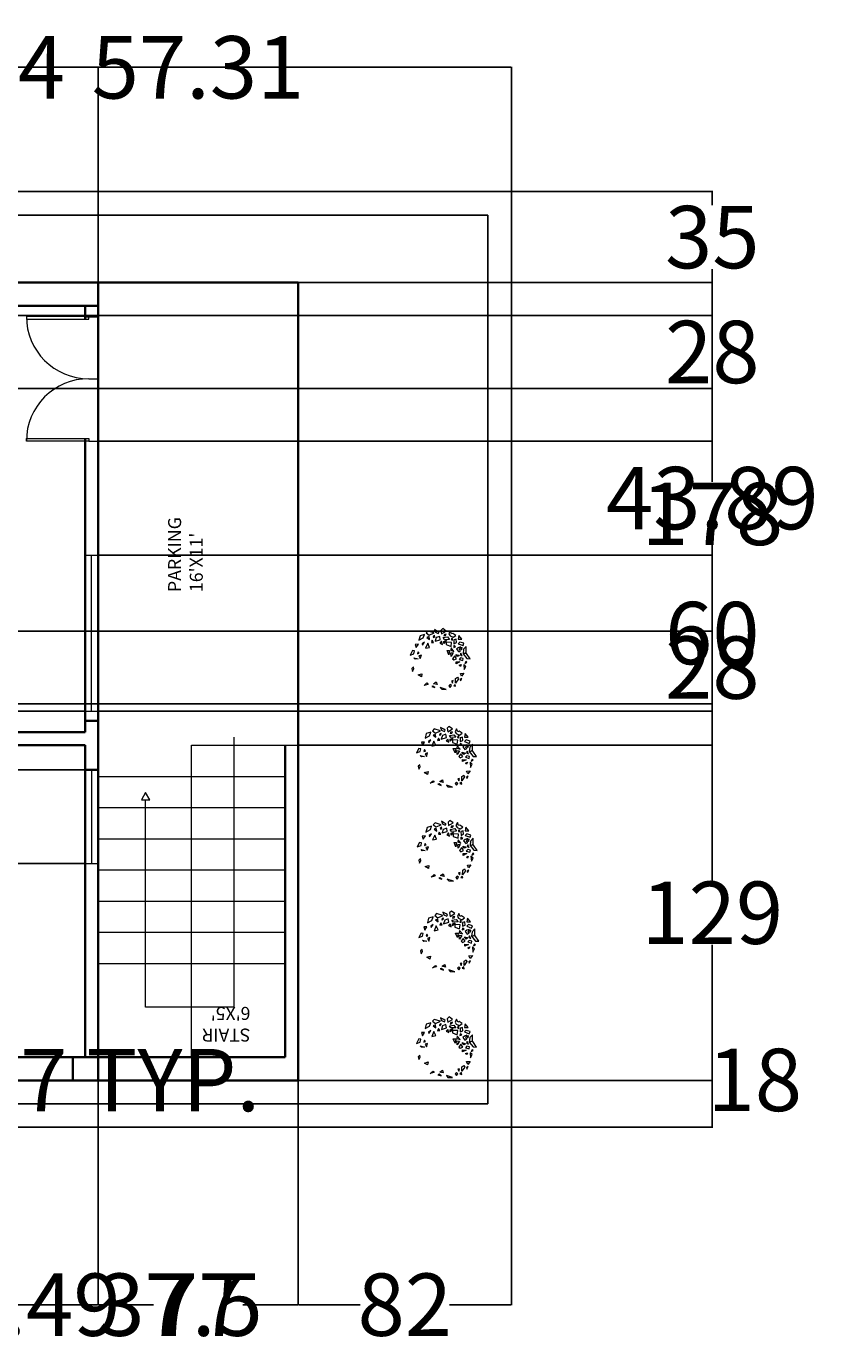
# Model space of a CAD drawing. Units: inches. Extents: x -1643 to -931, y 1907 to 2415.
# Tile 3 of 3: x -1236 to -931, y 1907 to 2415. Entities that reach past the tile are written whole.
import ezdxf

# ---------------------------------------------------------------- set-up
doc = ezdxf.new("R2010")
doc.units = ezdxf.units.IN
for name, color, linetype, lineweight in [('A-ANNO-DIMS', 2, 'Continuous', 18), ('A-AREA-IDEN', 7, 'Continuous', 18), ('A-DOOR', 3, 'Continuous', 18), ('A-FLOR-STRS', 7, 'Continuous', 18), ('A-GLAZ', 4, 'Continuous', 18), ('A-WALL', 7, 'Continuous', 35), ('C-PROP', 8, 'Continuous', 25), ('L-PLNT', 94, 'Continuous', 13)]:
    doc.layers.add(name, color=color, linetype=linetype, lineweight=lineweight)
doc.styles.get("Standard").update_dxf_attribs({"font": 'arial.ttf', "height": 24})
doc.dimstyles.get("Standard").update_dxf_attribs({"dimtxt": 0.18, "dimasz": 0.18, "dimexe": 0.18, "dimexo": 0.0625, "dimgap": 0.09, "dimtad": 0, "dimtih": 1, "dimtoh": 1, "dimdec": 4, "dimzin": 0, "dimdsep": 46, "dimtxsty": 'Standard', "dimcen": 0.09, "dimadec": 0, "dimazin": 0, "dimtfac": 1, "dimtdec": 4, "dimtofl": 0, "dimtmove": 0, "dimatfit": 3, "dimfxl": 1, "dimtolj": 1, "dimtzin": 0, "dimarcsym": 0})

# ---------------------------------------------------------------- blocks, each defined once
blk = doc.blocks.new('*U11')
for p, q in [((0, 5), (0, 0)), ((0, 2.5), (60, 2.5)), ((60, 5), (60, 0))]:
    blk.add_line(p, q)
blk = doc.blocks.new('*U4')
for p, q in [((0, 5), (0, 0)), ((0, 2.5), (36, 2.5)), ((36, 5), (36, 0))]:
    blk.add_line(p, q)
blk = doc.blocks.new('*U12')
for p, q in [((0, 0), (0, -6)), ((-40, 0), (-40, -6))]:
    blk.add_line(p, q)
blk.add_lwpolyline([(0, 0), (0, 40), (-1.75, 40), (-1.75, 0)], close=True)
blk.add_arc((0, 0), 40, 90, 180)
blk = doc.blocks.new('*U13')
for p, q in [((0, 0), (0, -6)), ((40, 0), (40, -6))]:
    blk.add_line(p, q)
blk.add_lwpolyline([(0, 0), (0, 40), (1.75, 40), (1.75, 0)], close=True)
blk.add_arc((0, 0), 40, 0, 90)
blk = doc.blocks.new('*U17')
for points in [[(-113, 281), (-131, 263), (-101, 241), (-53, 263)], [(-51, 296), (-41, 270), (-13, 257), (-5, 270), (-20, 278)], [(31, 305), (14, 287), (19, 254), (64, 281)], [(105, 283), (91, 254), (102, 235), (133, 221), (160, 239), (129, 259), (117, 254)], [(-207, 153), (-238, 151), (-229, 120)], [(-147, 248), (-191, 235), (-203, 191), (-159, 215)], [(-147, 173), (-169, 158), (-166, 144)], [(-116, 162), (-138, 114), (-99, 122)], [(-123, 219), (-97, 199), (-102, 228)], [(-73, 191), (-80, 169), (-58, 171)], [(-49, 241), (-63, 228), (-58, 217), (-46, 230)], [(1, 230), (-34, 217), (-44, 182), (7, 197)], [(19, 182), (2, 164), (28, 151)], [(35, 217), (79, 224), (97, 199), (49, 197)], [(66, 252), (47, 248), (42, 235), (59, 239)], [(43, 160), (43, 180), (67, 191), (54, 175)], [(64, 173), (64, 149), (112, 131), (117, 171)], [(117, 210), (115, 197), (126, 193), (126, 210)], [(139, 140), (138, 122), (157, 129)], [(163, 202), (139, 195), (141, 158), (165, 169)], [(189, 237), (181, 202), (217, 202)], [(199, 173), (182, 158), (229, 140), (237, 162)], [(261, 131), (234, 103), (229, 59), (266, 13), (299, 10), (263, 63), (237, 61), (261, 72)], [(-287, 46), (-250, 59), (-245, 87), (-265, 90)], [(-209, 10), (-239, 8), (-250, 21)], [(-209, 79), (-215, 59), (-200, 65)], [(-178, 46), (-202, 39), (-190, 13)], [(90, 48), (73, 90), (97, 90)], [(112, 116), (109, 94), (139, 83)], [(109, 70), (134, 68), (112, 32)], [(148, 39), (127, 10), (139, -1), (165, 10)], [(191, 43), (175, 32), (158, 54)], [(206, 127), (181, 118), (165, 105), (187, 79), (206, 90), (194, 98)], [(206, 19), (191, 4), (227, -7), (232, 13)], [(208, 65), (201, 52), (220, 39)], [(222, 120), (208, 116), (213, 98), (218, 103)], [(-255, -69), (-270, -84), (-265, -113), (-251, -89)], [(198, -20), (163, -38), (163, -18)], [(211, -45), (203, -64), (193, -53)], [(237, -45), (242, -95), (258, -64)], [(256, -16), (247, -34), (266, -23)], [(-210, -146), (-173, -135), (-178, -165)], [(-123, -225), (-113, -240), (-152, -249)], [(-65, -256), (-77, -260), (-46, -271)], [(-59, -234), (-32, -216), (-25, -242)], [(103, -240), (90, -253), (103, -269), (117, -251)], [(134, -203), (117, -207), (127, -227)], [(153, -240), (138, -253), (157, -258)], [(155, -227), (157, -183), (175, -170), (184, -187)], [(205, -205), (218, -181), (201, -192)], [(237, -130), (215, -159), (203, -132)], [(6, -269), (21, -286), (66, -289)]]:
    blk.add_lwpolyline(points, close=True)
blk = doc.blocks.new('*D19')
at = {"layer": 'A-ANNO-DIMS', "color": 0, "lineweight": -2, "transparency": 16777216}
for p, q in [((-1470.32, 2019.19), (-1470.32, 2009.1)), ((-1403.82, 2019.19), (-1403.82, 2009.1)), ((-1470.14, 2009.28), (-1404, 2009.28)), ((-1403.82, 2009.28), (-1403.64, 2009.28))]:
    blk.add_line(p, q, dxfattribs=at)
at = {"layer": 'A-ANNO-DIMS', "color": 0, "transparency": 16777216}
for points in [[(-1470.14, 2009.31), (-1470.14, 2009.25), (-1470.32, 2009.28)], [(-1404, 2009.31), (-1404, 2009.25), (-1403.82, 2009.28)]]:
    blk.add_solid(points, dxfattribs=at)
at = {"layer": 'Defpoints', "color": 0, "transparency": 16777216}
for p in [(-1470.32, 2019.25), (-1403.82, 2019.25), (-1403.82, 2009.28)]:
    blk.add_point(p, dxfattribs=at)
at = {"layer": 'A-ANNO-DIMS', "color": 0, "transparency": 16777216, "insert": (-1269.29, 2009.28), "char_height": 24, "attachment_point": 5}
blk.add_mtext('\\A1;BED SET 67 TYP.', dxfattribs=at)
blk = doc.blocks.new('*D21')
at = {"layer": 'A-ANNO-DIMS', "color": 0, "lineweight": -2, "transparency": 16777216}
for p, q in [((-1529.17, 2351.21), (-1529.17, 2399.16)), ((-1528.99, 2398.98), (-1316.21, 2398.98)), ((-1049.35, 2398.98), (-1262.12, 2398.98)), ((-1049.17, 2351.21), (-1049.17, 2399.16))]:
    blk.add_line(p, q, dxfattribs=at)
at = {"layer": 'A-ANNO-DIMS', "color": 0, "transparency": 16777216}
for points in [[(-1528.99, 2399.01), (-1528.99, 2398.95), (-1529.17, 2398.98)], [(-1049.35, 2399.01), (-1049.35, 2398.95), (-1049.17, 2398.98)]]:
    blk.add_solid(points, dxfattribs=at)
at = {"layer": 'Defpoints', "color": 0, "transparency": 16777216}
for p in [(-1049.17, 2398.98), (-1529.17, 2351.15), (-1049.17, 2351.15)]:
    blk.add_point(p, dxfattribs=at)
at = {"layer": 'A-ANNO-DIMS', "color": 0, "transparency": 16777216, "insert": (-1289.17, 2398.98), "char_height": 24, "attachment_point": 5}
blk.add_mtext('\\A1;480', dxfattribs=at)
blk = doc.blocks.new('*D26')
at = {"layer": 'A-ANNO-DIMS', "color": 0, "lineweight": -2, "transparency": 16777216}
for p, q in [((-1265.48, 2316.19), (-1265.48, 2399.16)), ((-1265.3, 2398.98), (-1208.35, 2398.98)), ((-1208.17, 2316.21), (-1208.17, 2399.16)), ((-1208.17, 2398.98), (-1207.99, 2398.98))]:
    blk.add_line(p, q, dxfattribs=at)
at = {"layer": 'A-ANNO-DIMS', "color": 0, "transparency": 16777216}
for points in [[(-1265.3, 2399.01), (-1265.3, 2398.95), (-1265.48, 2398.98)], [(-1208.35, 2399.01), (-1208.35, 2398.95), (-1208.17, 2398.98)]]:
    blk.add_solid(points, dxfattribs=at)
at = {"layer": 'Defpoints', "color": 0, "transparency": 16777216}
for p in [(-1208.17, 2398.98), (-1265.48, 2316.13), (-1208.17, 2316.15)]:
    blk.add_point(p, dxfattribs=at)
at = {"layer": 'A-ANNO-DIMS', "color": 0, "transparency": 16777216, "insert": (-1169.72, 2398.98), "char_height": 24, "attachment_point": 5}
blk.add_mtext('\\A1;57.31', dxfattribs=at)
blk = doc.blocks.new('*D27')
at = {"layer": 'A-ANNO-DIMS', "color": 0, "lineweight": -2, "transparency": 16777216}
for p, q in [((-1208.17, 2009.08), (-1208.17, 1922.66)), ((-1131.17, 2009.08), (-1131.17, 1922.66)), ((-1207.99, 1922.84), (-1186.85, 1922.84)), ((-1131.35, 1922.84), (-1152.49, 1922.84))]:
    blk.add_line(p, q, dxfattribs=at)
at = {"layer": 'A-ANNO-DIMS', "color": 0, "transparency": 16777216}
for points in [[(-1207.99, 1922.87), (-1207.99, 1922.81), (-1208.17, 1922.84)], [(-1131.35, 1922.87), (-1131.35, 1922.81), (-1131.17, 1922.84)]]:
    blk.add_solid(points, dxfattribs=at)
at = {"layer": 'Defpoints', "color": 0, "transparency": 16777216}
for p in [(-1208.17, 2009.15), (-1131.17, 2009.15), (-1131.17, 1922.84)]:
    blk.add_point(p, dxfattribs=at)
at = {"layer": 'A-ANNO-DIMS', "color": 0, "transparency": 16777216, "insert": (-1169.67, 1922.84), "char_height": 24, "attachment_point": 5}
blk.add_mtext('\\A1;77', dxfattribs=at)
blk = doc.blocks.new('*D28')
at = {"layer": 'A-ANNO-DIMS', "color": 0, "lineweight": -2, "transparency": 16777216}
for p, q in [((-1131.17, 2009.08), (-1131.17, 1922.66)), ((-1049.17, 1991.08), (-1049.17, 1922.66)), ((-1130.99, 1922.84), (-1107.34, 1922.84)), ((-1049.35, 1922.84), (-1072.99, 1922.84))]:
    blk.add_line(p, q, dxfattribs=at)
at = {"layer": 'A-ANNO-DIMS', "color": 0, "transparency": 16777216}
for points in [[(-1130.99, 1922.87), (-1130.99, 1922.81), (-1131.17, 1922.84)], [(-1049.35, 1922.87), (-1049.35, 1922.81), (-1049.17, 1922.84)]]:
    blk.add_solid(points, dxfattribs=at)
at = {"layer": 'Defpoints', "color": 0, "transparency": 16777216}
for p in [(-1131.17, 2009.15), (-1049.17, 1991.15), (-1049.17, 1922.84)]:
    blk.add_point(p, dxfattribs=at)
at = {"layer": 'A-ANNO-DIMS', "color": 0, "transparency": 16777216, "insert": (-1090.17, 1922.84), "char_height": 24, "attachment_point": 5}
blk.add_mtext('\\A1;82', dxfattribs=at)
blk = doc.blocks.new('*D29')
at = {"layer": 'A-ANNO-DIMS', "color": 0, "lineweight": -2, "transparency": 16777216}
for p, q in [((-1131.1, 2009.15), (-971.69, 2009.15)), ((-971.87, 2009.15), (-971.87, 2009.33)), ((-971.87, 2009.33), (-971.69, 2009.33)), ((-971.87, 1991.33), (-971.87, 2008.97)), ((-1049.1, 1991.15), (-971.69, 1991.15))]:
    blk.add_line(p, q, dxfattribs=at)
at = {"layer": 'A-ANNO-DIMS', "color": 0, "transparency": 16777216}
for points in [[(-971.9, 2008.97), (-971.84, 2008.97), (-971.87, 2009.15)], [(-971.9, 1991.33), (-971.84, 1991.33), (-971.87, 1991.15)]]:
    blk.add_solid(points, dxfattribs=at)
at = {"layer": 'Defpoints', "color": 0, "transparency": 16777216}
for p in [(-1131.17, 2009.15), (-971.87, 2009.15), (-1049.17, 1991.15)]:
    blk.add_point(p, dxfattribs=at)
at = {"layer": 'A-ANNO-DIMS', "color": 0, "transparency": 16777216, "insert": (-955.51, 2009.33), "char_height": 24, "attachment_point": 5}
blk.add_mtext('\\A1;18', dxfattribs=at)
blk = doc.blocks.new('*D30')
at = {"layer": 'A-ANNO-DIMS', "color": 0, "lineweight": -2, "transparency": 16777216}
for p, q in [((-1131.1, 2138.15), (-971.69, 2138.15)), ((-971.87, 2137.97), (-971.87, 2085.99)), ((-971.87, 2009.33), (-971.87, 2061.3)), ((-1131.1, 2009.15), (-971.69, 2009.15))]:
    blk.add_line(p, q, dxfattribs=at)
at = {"layer": 'A-ANNO-DIMS', "color": 0, "transparency": 16777216}
for points in [[(-971.9, 2137.97), (-971.84, 2137.97), (-971.87, 2138.15)], [(-971.9, 2009.33), (-971.84, 2009.33), (-971.87, 2009.15)]]:
    blk.add_solid(points, dxfattribs=at)
at = {"layer": 'Defpoints', "color": 0, "transparency": 16777216}
for p in [(-1131.17, 2138.15), (-971.87, 2138.15), (-1131.17, 2009.15)]:
    blk.add_point(p, dxfattribs=at)
at = {"layer": 'A-ANNO-DIMS', "color": 0, "transparency": 16777216, "insert": (-971.87, 2073.65), "char_height": 24, "attachment_point": 5}
blk.add_mtext('\\A1;129', dxfattribs=at)
blk = doc.blocks.new('*D31')
at = {"layer": 'A-ANNO-DIMS', "color": 0, "lineweight": -2, "transparency": 16777216}
for p, q in [((-1131.1, 2316.15), (-971.69, 2316.15)), ((-971.87, 2315.97), (-971.87, 2239.49)), ((-971.87, 2138.33), (-971.87, 2214.8)), ((-1131.1, 2138.15), (-971.69, 2138.15))]:
    blk.add_line(p, q, dxfattribs=at)
at = {"layer": 'A-ANNO-DIMS', "color": 0, "transparency": 16777216}
for points in [[(-971.9, 2315.97), (-971.84, 2315.97), (-971.87, 2316.15)], [(-971.9, 2138.33), (-971.84, 2138.33), (-971.87, 2138.15)]]:
    blk.add_solid(points, dxfattribs=at)
at = {"layer": 'Defpoints', "color": 0, "transparency": 16777216}
for p in [(-1131.17, 2316.15), (-971.87, 2316.15), (-1131.17, 2138.15)]:
    blk.add_point(p, dxfattribs=at)
at = {"layer": 'A-ANNO-DIMS', "color": 0, "transparency": 16777216, "insert": (-971.87, 2227.15), "char_height": 24, "attachment_point": 5}
blk.add_mtext('\\A1;178', dxfattribs=at)
blk = doc.blocks.new('*D32')
at = {"layer": 'A-ANNO-DIMS', "color": 0, "lineweight": -2, "transparency": 16777216}
for p, q in [((-1049.1, 2351.15), (-971.69, 2351.15)), ((-971.87, 2350.97), (-971.87, 2346)), ((-971.87, 2316.33), (-971.87, 2321.29)), ((-1131.1, 2316.15), (-971.69, 2316.15))]:
    blk.add_line(p, q, dxfattribs=at)
at = {"layer": 'A-ANNO-DIMS', "color": 0, "transparency": 16777216}
for points in [[(-971.9, 2350.97), (-971.84, 2350.97), (-971.87, 2351.15)], [(-971.9, 2316.33), (-971.84, 2316.33), (-971.87, 2316.15)]]:
    blk.add_solid(points, dxfattribs=at)
at = {"layer": 'Defpoints', "color": 0, "transparency": 16777216}
for p in [(-1049.17, 2351.15), (-971.87, 2351.15), (-1131.17, 2316.15)]:
    blk.add_point(p, dxfattribs=at)
at = {"layer": 'A-ANNO-DIMS', "color": 0, "transparency": 16777216, "insert": (-971.87, 2333.65), "char_height": 24, "attachment_point": 5}
blk.add_mtext('\\A1;35', dxfattribs=at)
blk = doc.blocks.new('*D39')
at = {"layer": 'A-ANNO-DIMS', "color": 0, "lineweight": -2, "transparency": 16777216}
for p, q in [((-1328.16, 2009.1), (-1328.16, 1922.66)), ((-1281.67, 2009.06), (-1281.67, 1922.66)), ((-1327.98, 1922.84), (-1281.85, 1922.84)), ((-1281.67, 1922.84), (-1281.49, 1922.84))]:
    blk.add_line(p, q, dxfattribs=at)
at = {"layer": 'A-ANNO-DIMS', "color": 0, "transparency": 16777216}
for points in [[(-1327.98, 1922.87), (-1327.98, 1922.81), (-1328.16, 1922.84)], [(-1281.85, 1922.87), (-1281.85, 1922.81), (-1281.67, 1922.84)]]:
    blk.add_solid(points, dxfattribs=at)
at = {"layer": 'Defpoints', "color": 0, "transparency": 16777216}
for p in [(-1328.16, 2009.16), (-1281.67, 2009.13), (-1281.67, 1922.84)]:
    blk.add_point(p, dxfattribs=at)
at = {"layer": 'A-ANNO-DIMS', "color": 0, "transparency": 16777216, "insert": (-1240.4, 1922.84), "char_height": 24, "attachment_point": 5}
blk.add_mtext('\\A1;46.49', dxfattribs=at)
blk = doc.blocks.new('*D42')
at = {"layer": 'A-ANNO-DIMS', "color": 0, "lineweight": -2, "transparency": 16777216}
for p, q in [((-1208.08, 2255.15), (-971.69, 2255.15)), ((-971.87, 2254.97), (-971.87, 2245.56)), ((-971.87, 2211.44), (-971.87, 2220.85)), ((-1208.11, 2211.26), (-971.69, 2211.26))]:
    blk.add_line(p, q, dxfattribs=at)
at = {"layer": 'A-ANNO-DIMS', "color": 0, "transparency": 16777216}
for points in [[(-971.9, 2254.97), (-971.84, 2254.97), (-971.87, 2255.15)], [(-971.9, 2211.44), (-971.84, 2211.44), (-971.87, 2211.26)]]:
    blk.add_solid(points, dxfattribs=at)
at = {"layer": 'Defpoints', "color": 0, "transparency": 16777216}
for p in [(-1208.14, 2255.15), (-1208.18, 2211.26), (-971.87, 2211.26)]:
    blk.add_point(p, dxfattribs=at)
at = {"layer": 'A-ANNO-DIMS', "color": 0, "transparency": 16777216, "insert": (-971.87, 2233.21), "char_height": 24, "attachment_point": 5}
blk.add_mtext('\\A1;43.89', dxfattribs=at)
blk = doc.blocks.new('*D43')
at = {"layer": 'A-ANNO-DIMS', "color": 0, "lineweight": -2, "transparency": 16777216}
for p, q in [((-1208.11, 2211.26), (-971.69, 2211.26)), ((-971.87, 2211.08), (-971.87, 2193.6)), ((-971.87, 2151.44), (-971.87, 2168.92)), ((-1208.11, 2151.26), (-971.69, 2151.26))]:
    blk.add_line(p, q, dxfattribs=at)
at = {"layer": 'A-ANNO-DIMS', "color": 0, "transparency": 16777216}
for points in [[(-971.9, 2211.08), (-971.84, 2211.08), (-971.87, 2211.26)], [(-971.9, 2151.44), (-971.84, 2151.44), (-971.87, 2151.26)]]:
    blk.add_solid(points, dxfattribs=at)
at = {"layer": 'Defpoints', "color": 0, "transparency": 16777216}
for p in [(-1208.18, 2211.26), (-1208.18, 2151.26), (-971.87, 2151.26)]:
    blk.add_point(p, dxfattribs=at)
at = {"layer": 'A-ANNO-DIMS', "color": 0, "transparency": 16777216, "insert": (-971.87, 2181.26), "char_height": 24, "attachment_point": 5}
blk.add_mtext('\\A1;60', dxfattribs=at)
blk = doc.blocks.new('*D44')
at = {"layer": 'A-ANNO-DIMS', "color": 0, "lineweight": -2, "transparency": 16777216}
for p, q in [((-1213.24, 2151.26), (-1561.32, 2151.26)), ((-1561.14, 2151.08), (-1561.14, 2128.82)), ((-1213.11, 2128.64), (-1561.32, 2128.64)), ((-1561.14, 2128.46), (-1561.32, 2128.46)), ((-1561.14, 2128.64), (-1561.14, 2128.46))]:
    blk.add_line(p, q, dxfattribs=at)
at = {"layer": 'A-ANNO-DIMS', "color": 0, "transparency": 16777216}
for points in [[(-1561.17, 2151.08), (-1561.11, 2151.08), (-1561.14, 2151.26)], [(-1561.17, 2128.82), (-1561.11, 2128.82), (-1561.14, 2128.64)]]:
    blk.add_solid(points, dxfattribs=at)
at = {"layer": 'Defpoints', "color": 0, "transparency": 16777216}
for p in [(-1213.18, 2151.26), (-1561.14, 2128.64), (-1213.05, 2128.64)]:
    blk.add_point(p, dxfattribs=at)
at = {"layer": 'A-ANNO-DIMS', "color": 0, "transparency": 16777216, "insert": (-1601.99, 2128.46), "char_height": 24, "attachment_point": 5}
blk.add_mtext('\\A1;22.62', dxfattribs=at)
blk = doc.blocks.new('*D45')
at = {"layer": 'A-ANNO-DIMS', "color": 0, "lineweight": -2, "transparency": 16777216}
for p, q in [((-1213.11, 2128.64), (-1561.32, 2128.64)), ((-1561.14, 2128.46), (-1561.14, 2122.99)), ((-1561.14, 2092.82), (-1561.14, 2098.29)), ((-1213.11, 2092.64), (-1561.32, 2092.64))]:
    blk.add_line(p, q, dxfattribs=at)
at = {"layer": 'A-ANNO-DIMS', "color": 0, "transparency": 16777216}
for points in [[(-1561.17, 2128.46), (-1561.11, 2128.46), (-1561.14, 2128.64)], [(-1561.17, 2092.82), (-1561.11, 2092.82), (-1561.14, 2092.64)]]:
    blk.add_solid(points, dxfattribs=at)
at = {"layer": 'Defpoints', "color": 0, "transparency": 16777216}
for p in [(-1213.05, 2128.64), (-1561.14, 2092.64), (-1213.05, 2092.64)]:
    blk.add_point(p, dxfattribs=at)
at = {"layer": 'A-ANNO-DIMS', "color": 0, "transparency": 16777216, "insert": (-1561.14, 2110.64), "char_height": 24, "attachment_point": 5}
blk.add_mtext('\\A1;36', dxfattribs=at)
blk = doc.blocks.new('*D46')
at = {"layer": 'A-ANNO-DIMS', "color": 0, "lineweight": -2, "transparency": 16777216}
for p, q in [((-1213.11, 2092.64), (-1561.32, 2092.64)), ((-1561.14, 2092.46), (-1561.14, 2067.69)), ((-1561.14, 2018.33), (-1561.14, 2043.1)), ((-1213.23, 2018.15), (-1561.32, 2018.15))]:
    blk.add_line(p, q, dxfattribs=at)
at = {"layer": 'A-ANNO-DIMS', "color": 0, "transparency": 16777216}
for points in [[(-1561.17, 2092.46), (-1561.11, 2092.46), (-1561.14, 2092.64)], [(-1561.17, 2018.33), (-1561.11, 2018.33), (-1561.14, 2018.15)]]:
    blk.add_solid(points, dxfattribs=at)
at = {"layer": 'Defpoints', "color": 0, "transparency": 16777216}
for p in [(-1213.05, 2092.64), (-1561.14, 2018.15), (-1213.17, 2018.15)]:
    blk.add_point(p, dxfattribs=at)
at = {"layer": 'A-ANNO-DIMS', "color": 0, "transparency": 16777216, "insert": (-1561.14, 2055.39), "char_height": 24, "attachment_point": 5}
blk.add_mtext('\\A1;74.5', dxfattribs=at)
blk = doc.blocks.new('*D54')
at = {"layer": 'A-ANNO-DIMS', "color": 0, "lineweight": -2, "transparency": 16777216}
for p, q in [((-1438.11, 2303.44), (-971.69, 2303.44)), ((-971.87, 2303.26), (-971.87, 2301.79)), ((-1438.11, 2275.44), (-971.69, 2275.44)), ((-971.87, 2275.62), (-971.87, 2277.1))]:
    blk.add_line(p, q, dxfattribs=at)
at = {"layer": 'A-ANNO-DIMS', "color": 0, "transparency": 16777216}
for points in [[(-971.9, 2303.26), (-971.84, 2303.26), (-971.87, 2303.44)], [(-971.9, 2275.62), (-971.84, 2275.62), (-971.87, 2275.44)]]:
    blk.add_solid(points, dxfattribs=at)
at = {"layer": 'Defpoints', "color": 0, "transparency": 16777216}
for p in [(-1438.17, 2303.44), (-1438.17, 2275.44), (-971.87, 2275.44)]:
    blk.add_point(p, dxfattribs=at)
at = {"layer": 'A-ANNO-DIMS', "color": 0, "transparency": 16777216, "insert": (-971.87, 2289.44), "char_height": 24, "attachment_point": 5}
blk.add_mtext('\\A1;28', dxfattribs=at)
blk = doc.blocks.new('*D56')
at = {"layer": 'A-ANNO-DIMS', "color": 0, "lineweight": -2, "transparency": 16777216}
for p, q in [((-1425.11, 2182), (-971.69, 2182)), ((-971.87, 2181.82), (-971.87, 2180.35)), ((-1424.39, 2154), (-971.69, 2154)), ((-971.87, 2154.18), (-971.87, 2155.66))]:
    blk.add_line(p, q, dxfattribs=at)
at = {"layer": 'A-ANNO-DIMS', "color": 0, "transparency": 16777216}
for points in [[(-971.9, 2181.82), (-971.84, 2181.82), (-971.87, 2182)], [(-971.9, 2154.18), (-971.84, 2154.18), (-971.87, 2154)]]:
    blk.add_solid(points, dxfattribs=at)
at = {"layer": 'Defpoints', "color": 0, "transparency": 16777216}
for p in [(-1425.17, 2182), (-1424.45, 2154), (-971.87, 2154)]:
    blk.add_point(p, dxfattribs=at)
at = {"layer": 'A-ANNO-DIMS', "color": 0, "transparency": 16777216, "insert": (-971.87, 2168), "char_height": 24, "attachment_point": 5}
blk.add_mtext('\\A1;28', dxfattribs=at)
blk = doc.blocks.new('*D59')
at = {"layer": 'A-ANNO-DIMS', "color": 0, "lineweight": -2, "transparency": 16777216}
for p, q in [((-1366.66, 2143.21), (-1366.66, 2399.16)), ((-1366.48, 2398.98), (-1302.71, 2398.98)), ((-1302.53, 2143.21), (-1302.53, 2399.16)), ((-1302.53, 2398.98), (-1302.35, 2398.98))]:
    blk.add_line(p, q, dxfattribs=at)
at = {"layer": 'A-ANNO-DIMS', "color": 0, "transparency": 16777216}
for points in [[(-1366.48, 2399.01), (-1366.48, 2398.95), (-1366.66, 2398.98)], [(-1302.71, 2399.01), (-1302.71, 2398.95), (-1302.53, 2398.98)]]:
    blk.add_solid(points, dxfattribs=at)
at = {"layer": 'Defpoints', "color": 0, "transparency": 16777216}
for p in [(-1302.53, 2398.98), (-1366.66, 2143.15), (-1302.53, 2143.15)]:
    blk.add_point(p, dxfattribs=at)
at = {"layer": 'A-ANNO-DIMS', "color": 0, "transparency": 16777216, "insert": (-1261.75, 2398.98), "char_height": 24, "attachment_point": 5}
blk.add_mtext('\\A1;64.14', dxfattribs=at)
blk = doc.blocks.new('*D63')
at = {"layer": 'A-ANNO-DIMS', "color": 0, "lineweight": -2, "transparency": 16777216}
for p, q in [((-1245.67, 2009.06), (-1245.67, 1922.66)), ((-1208.17, 2009.08), (-1208.17, 1922.66)), ((-1245.49, 1922.84), (-1208.35, 1922.84)), ((-1208.17, 1922.84), (-1207.99, 1922.84))]:
    blk.add_line(p, q, dxfattribs=at)
at = {"layer": 'A-ANNO-DIMS', "color": 0, "transparency": 16777216}
for points in [[(-1245.49, 1922.87), (-1245.49, 1922.81), (-1245.67, 1922.84)], [(-1208.35, 1922.87), (-1208.35, 1922.81), (-1208.17, 1922.84)]]:
    blk.add_solid(points, dxfattribs=at)
at = {"layer": 'Defpoints', "color": 0, "transparency": 16777216}
for p in [(-1245.67, 2009.13), (-1208.17, 2009.15), (-1208.17, 1922.84)]:
    blk.add_point(p, dxfattribs=at)
at = {"layer": 'A-ANNO-DIMS', "color": 0, "transparency": 16777216, "insert": (-1176.64, 1922.84), "char_height": 24, "attachment_point": 5}
blk.add_mtext('\\A1;37.5', dxfattribs=at)

msp = doc.modelspace()

# ---------------------------------------------------------------- linework, layer by layer
at = {"layer": 'A-FLOR-STRS'}
for p, q in [((-1172.1668, 2138.1464), (-1131.1668, 2138.1464)), ((-1172.1668, 2018.1464), (-1172.1668, 2138.1464)), ((-1155.9057, 2141.227), (-1155.9057, 2037.3635)), ((-1208.1668, 2126.1464), (-1136.1668, 2126.1464)), ((-1189.8704, 2119.8826), (-1191.4662, 2117.0695)), ((-1191.4662, 2117.0695), (-1188.2691, 2117.0695)), ((-1188.2691, 2117.0695), (-1189.8704, 2119.8826)), ((-1189.8704, 2116.6774), (-1189.8704, 2117.0695)), ((-1208.1668, 2114.1464), (-1136.1668, 2114.1464)), ((-1189.8704, 2037.3635), (-1189.8704, 2116.6774)), ((-1208.1668, 2102.1464), (-1136.1668, 2102.1464)), ((-1208.1668, 2090.1464), (-1136.1668, 2090.1464)), ((-1208.1668, 2078.1464), (-1136.1668, 2078.1464)), ((-1208.1668, 2066.1464), (-1136.1668, 2066.1464)), ((-1208.1668, 2054.1464), (-1136.1668, 2054.1464)), ((-1155.9057, 2037.3635), (-1189.8704, 2037.3635))]:
    msp.add_line(p, q, dxfattribs=at)
at = {"layer": 'A-WALL'}
for p, q in [((-1511.1668, 2316.1464), (-1131.1668, 2316.1464)), ((-1208.1668, 2307.1464), (-1208.1668, 2316.1464)), ((-1131.1668, 2138.1464), (-1131.1668, 2316.1464)), ((-1502.1668, 2307.1464), (-1213.1668, 2307.1464)), ((-1213.1668, 2307.1464), (-1208.1668, 2307.1464)), ((-1213.1668, 2302.1027), (-1213.1668, 2307.1464)), ((-1208.1668, 2143.1464), (-1208.1668, 2307.1464)), ((-1213.1668, 2303.1464), (-1208.1668, 2303.1464)), ((-1213.1668, 2279.1105), (-1213.1668, 2279.195)), ((-1213.1668, 2143.1464), (-1213.1668, 2256.2027)), ((-1208.1668, 2138.1464), (-1208.1668, 2154.2502)), ((-1213.1668, 2147.4503), (-1208.1668, 2147.4503)), ((-1302.5278, 2143.1464), (-1213.1668, 2143.1464)), ((-1291.1668, 2138.1464), (-1213.1668, 2138.1464)), ((-1213.1668, 2018.1464), (-1213.1668, 2138.1464)), ((-1208.1668, 2018.1464), (-1208.1668, 2138.1464)), ((-1136.1668, 2018.1464), (-1136.1668, 2138.1464)), ((-1131.1668, 2018.1464), (-1131.1668, 2138.1464)), ((-1213.1668, 2128.6553), (-1208.1668, 2128.6553)), ((-1377.1668, 2018.1464), (-1136.1668, 2018.1464)), ((-1217.8527, 2018.1464), (-1217.8527, 2009.1464)), ((-1208.1668, 2018.1464), (-1208.1668, 2009.1464)), ((-1131.1668, 2018.1464), (-1131.1668, 2009.1464)), ((-1511.1668, 2009.1464), (-1131.1668, 2009.1464))]:
    msp.add_line(p, q, dxfattribs=at)
at = {"layer": 'C-PROP'}
for p, q in [((-1529.1668, 2351.1464), (-1049.1668, 2351.1464)), ((-1049.1668, 2351.1464), (-1049.1668, 1991.1464)), ((-1520.1668, 2342.1464), (-1058.1668, 2342.1464)), ((-1058.1668, 2342.1464), (-1058.1668, 2000.1464)), ((-1520.1668, 2000.1464), (-1058.1668, 2000.1464)), ((-1529.1668, 1991.1464), (-1049.1668, 1991.1464))]:
    msp.add_line(p, q, dxfattribs=at)

# ---------------------------------------------------------------- block references
at = {"layer": 'A-DOOR', "xscale": 0.6, "yscale": 0.6, "zscale": 0.6, "rotation": 90.00000000000007}
for name, p in [('*U12', (-1211.7435, 2303.1527)), ('*U13', (-1211.7435, 2255.1527))]:
    msp.add_blockref(name, p, dxfattribs=at)
at = {"layer": 'A-GLAZ'}
for name, p, rotation in [('*U11', (-1208.1766, 2151.2595), 90.00000000000007), ('*U4', (-1208.047, 2092.64), 89.99999999999999)]:
    msp.add_blockref(name, p, dxfattribs=dict(at, rotation=rotation))
at = {"layer": 'L-PLNT', "xscale": 0.0393700787401575, "yscale": 0.0393700787401575, "zscale": 0.0393700787401575}
for p in [(-1076.7918, 2170.9662), (-1074.3848, 2133.327), (-1074.0839, 2097.1934), (-1073.4822, 2062.2642), (-1074.3791, 2021.5729)]:
    msp.add_blockref('*U17', p, dxfattribs=at)

# ---------------------------------------------------------------- texts
at = {"layer": 'A-AREA-IDEN', "char_height": 5, "attachment_point": 1}
for s, width, insert, rotation in [("PARKING\\P16'X11'", 21.970284, (-1181.2175, 2197.0541), 90), ("STAIR\\P6'X5'", 48.444606, (-1149.536, 2024.081), 180)]:
    msp.add_mtext_dynamic_manual_height_columns(s, width=width, gutter_width=120, heights=[0], dxfattribs=dict(at, insert=insert, rotation=rotation))

# ---------------------------------------------------------------- dimensions: what is measured, and where the dimension line sits
at = {"layer": 'A-ANNO-DIMS'}
for base, p1, p2, override, picture, middle in [((-1049.1668, 2398.9832), (-1529.1668, 2351.1464), (-1049.1668, 2351.1464), {"dimdec": 0, "dimlfac": 1, "dimrnd": 0, "dimzin": 0, "dimdsep": 46, "dimlunit": 2}, '*D21', (-1289.1668, 2398.9832)), ((-1302.5278, 2398.9832), (-1366.6634, 2143.1464), (-1302.5278, 2143.1464), {"dimdec": 2, "dimlfac": 1, "dimrnd": 0, "dimzin": 0, "dimdsep": 46, "dimlunit": 2}, '*D59', (-1261.7476, 2398.9832)), ((-1208.1668, 2398.9832), (-1265.4771, 2316.1314), (-1208.1668, 2316.1464), {"dimdec": 2, "dimlfac": 1, "dimrnd": 0, "dimzin": 0, "dimdsep": 46, "dimlunit": 2}, '*D26', (-1169.7195, 2398.9832)), ((-1281.6674, 1922.8359), (-1328.1588, 2009.1602), (-1281.6674, 2009.1256), {"dimdec": 2, "dimlfac": 1, "dimrnd": 0, "dimzin": 0, "dimdsep": 46, "dimlunit": 2}, '*D39', (-1240.396, 1922.8359)), ((-1208.1668, 1922.8359), (-1245.6674, 2009.1256), (-1208.1668, 2009.1464), {"dimdec": 1, "dimlfac": 1, "dimrnd": 0, "dimzin": 0, "dimdsep": 46, "dimlunit": 2}, '*D63', (-1176.6445, 1922.8359)), ((-1131.1668, 1922.8359), (-1208.1668, 2009.1464), (-1131.1668, 2009.1464), {"dimdec": 0, "dimlfac": 1, "dimrnd": 0, "dimzin": 0, "dimdsep": 46, "dimlunit": 2}, '*D27', (-1169.6668, 1922.8359)), ((-1049.1668, 1922.8359), (-1131.1668, 2009.1464), (-1049.1668, 1991.1464), {"dimdec": 0, "dimlfac": 1, "dimrnd": 0, "dimzin": 0, "dimdsep": 46, "dimlunit": 2}, '*D28', (-1090.1668, 1922.8359))]:
    dim = msp.add_linear_dim(base=base, p1=p1, p2=p2, dimstyle='Standard', override=override, dxfattribs=at)
    dim.commit()
    dim.dimension.update_dxf_attribs({"geometry": picture, "text_midpoint": middle})
for base, p1, p2, override, picture, middle in [((-971.8662, 2351.1464), (-1131.1668, 2316.1464), (-1049.1668, 2351.1464), {"dimdec": 0, "dimlfac": 1, "dimrnd": 0, "dimzin": 0, "dimdsep": 46, "dimlunit": 2}, '*D32', (-971.8662, 2333.6464)), ((-971.8662, 2316.1464), (-1131.1668, 2138.1464), (-1131.1668, 2316.1464), {"dimdec": 0, "dimlfac": 1, "dimrnd": 0, "dimzin": 0, "dimdsep": 46, "dimlunit": 2}, '*D31', (-971.8662, 2227.1464)), ((-971.8662, 2275.4425), (-1438.1708, 2303.4425), (-1438.1708, 2275.4425), {"dimdec": 0, "dimlfac": 1, "dimrnd": 0, "dimzin": 0, "dimdsep": 46, "dimlunit": 2}, '*D54', (-971.8662, 2289.4425)), ((-971.8662, 2211.2595), (-1208.1435, 2255.1527), (-1208.1766, 2211.2595), {"dimdec": 2, "dimlfac": 1, "dimrnd": 0, "dimzin": 0, "dimdsep": 46, "dimlunit": 2}, '*D42', (-971.8662, 2233.2061)), ((-971.8662, 2151.2595), (-1208.1766, 2211.2595), (-1208.1766, 2151.2595), {"dimdec": 0, "dimlfac": 1, "dimrnd": 0, "dimzin": 0, "dimdsep": 46, "dimlunit": 2}, '*D43', (-971.8662, 2181.2595)), ((-971.8662, 2154.0034), (-1425.1708, 2182.0034), (-1424.4498, 2154.0034), {"dimdec": 0, "dimlfac": 1, "dimrnd": 0, "dimzin": 0, "dimdsep": 46, "dimlunit": 2}, '*D56', (-971.8662, 2168.0034)), ((-1561.1409, 2128.64), (-1213.1766, 2151.2595), (-1213.047, 2128.64), {"dimdec": 2, "dimlfac": 1, "dimrnd": 0, "dimzin": 0, "dimdsep": 46, "dimlunit": 2}, '*D44', (-1601.9867, 2128.46)), ((-971.8662, 2138.1464), (-1131.1668, 2009.1464), (-1131.1668, 2138.1464), {"dimdec": 0, "dimlfac": 1, "dimrnd": 0, "dimzin": 0, "dimdsep": 46, "dimlunit": 2}, '*D30', (-971.8662, 2073.6464)), ((-1561.1409, 2092.64), (-1213.047, 2128.64), (-1213.047, 2092.64), {"dimdec": 0, "dimlfac": 1, "dimrnd": 0, "dimzin": 0, "dimdsep": 46, "dimlunit": 2}, '*D45', (-1561.1409, 2110.64)), ((-1561.1409, 2018.1464), (-1213.047, 2092.64), (-1213.1668, 2018.1464), {"dimdec": 1, "dimlfac": 1, "dimrnd": 0, "dimzin": 0, "dimdsep": 46, "dimlunit": 2}, '*D46', (-1561.1409, 2055.3932)), ((-971.8662, 2009.1464), (-1049.1668, 1991.1464), (-1131.1668, 2009.1464), {"dimdec": 0, "dimlfac": 1, "dimrnd": 0, "dimzin": 0, "dimdsep": 46, "dimlunit": 2}, '*D29', (-955.5116, 2009.3264))]:
    dim = msp.add_linear_dim(base=base, p1=p1, p2=p2, angle=90, dimstyle='Standard', override=override, dxfattribs=at)
    dim.commit()
    dim.dimension.update_dxf_attribs({"geometry": picture, "text_midpoint": middle})
dim = msp.add_linear_dim(base=(-1403.8243, 2009.277), p1=(-1470.3248, 2019.2521), p2=(-1403.8243, 2019.2521), text='BED SET <> TYP.', dimstyle='Standard', override={"dimdec": 0, "dimlfac": 1, "dimrnd": 0, "dimzin": 0, "dimdsep": 46, "dimlunit": 2}, dxfattribs=at)
dim.commit()
dim.dimension.update_dxf_attribs({"geometry": '*D19', "text_midpoint": (-1269.2869, 2009.277)})

doc.saveas('drawing.dxf')
